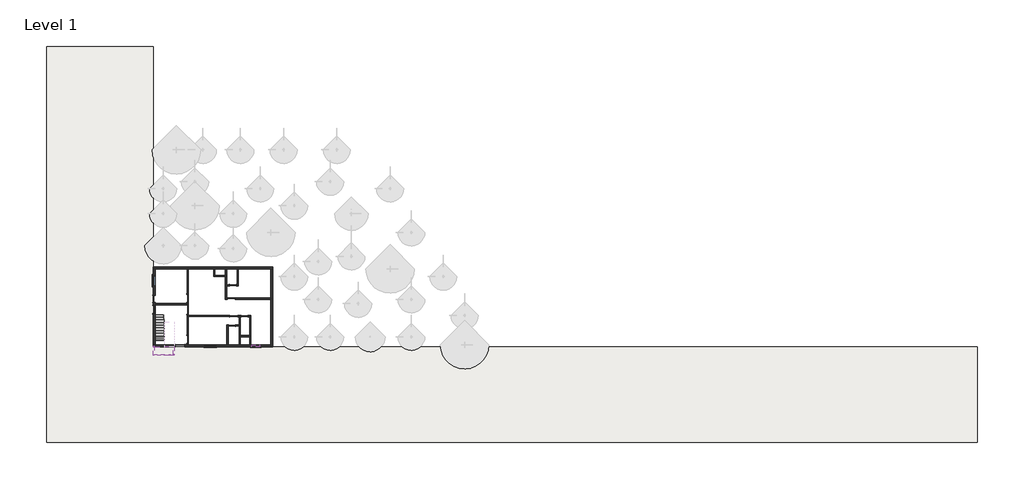
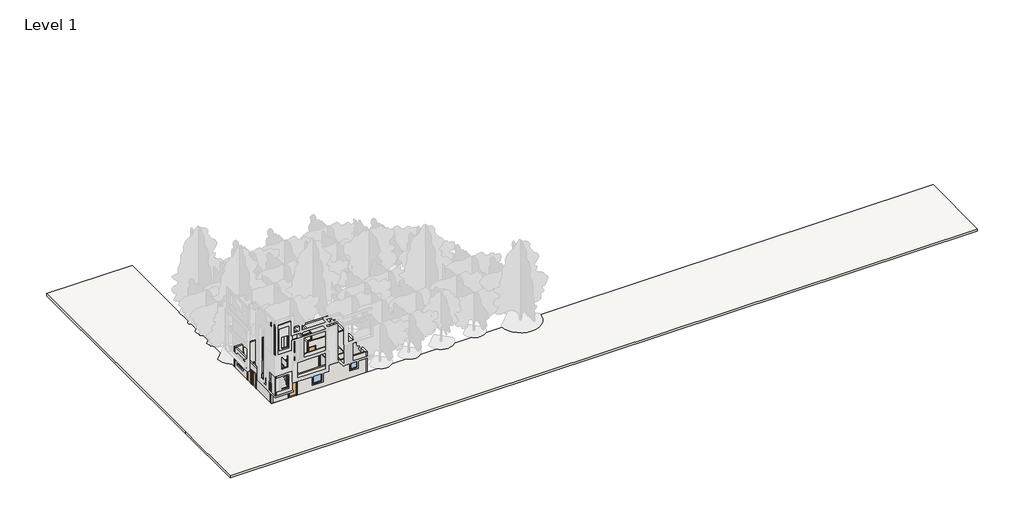
# One storey, part 1 of 2: 24 walls, 11 doors, 4 windows, 2 slabs, 1 stair flight.
"""IFC4 building model written with IfcOpenShell, lengths in millimetres."""

from ifc_helpers import new_model, si_unit, frame, origin, origin_with_axes, place, context, project, spatial, polyline, outline, extrude, faceted_brep, transform, mapped, element, save
from components import door_1fe7f57d, door_85036156, door_a3eb833a, door_a1797ceb, door_a90ba1ad, door_4f94b823, door_0848dd25, window_6c5853a0, window_f887c457, window_76f305d9

model = new_model("IFC4")

# Units and contexts
model_context = context("Model", 3, world=origin())
ifc_project = project(units=[si_unit("LENGTHUNIT", "METRE", prefix="MILLI")], contexts=[model_context])

# Site, building, storey
site = spatial("IfcSite", under=ifc_project)
building = spatial("IfcBuilding", under=site)
storey = spatial("IfcBuildingStorey", under=building, Name="Level 1", Elevation=0.0)

# Doors
placement = place(None, origin())
door_shape = door_1fe7f57d(model_context)
element("IfcDoor", 1, ObjectType="Single-Flush : 30\" x 80\"", at=placement, inside=storey, context=model_context, shape_type="MappedRepresentation", body=[
    mapped(door_shape, transform((-1197.7394758, 10653.5495492, 0.0), x_axis=(1.0, 0.0, 0.0), y_axis=(0.0, 1.0, 0.0), z_axis=(0.0, 0.0, 1.0))),
])
element("IfcDoor", 2, ObjectType="Single-Flush : 30\" x 80\"", at=placement, inside=storey, context=model_context, shape_type="MappedRepresentation", body=[
    mapped(door_shape, transform((135.7605242, 7148.3495492, 0.0), x_axis=(-1.0, 0.0, 0.0), y_axis=(0.0, -1.0, 0.0), z_axis=(0.0, 0.0, 1.0))),
])
element("IfcDoor", 3, ObjectType="Single-Flush : 30\" x 80\"", at=placement, inside=storey, context=model_context, shape_type="MappedRepresentation", body=[
    mapped(door_shape, transform((-1324.7394758, 6056.1495492, 0.0), x_axis=(-1.0, 0.0, 0.0), y_axis=(0.0, -1.0, 0.0), z_axis=(0.0, 0.0, 1.0))),
])
door_2_shape = door_85036156(model_context)
element("IfcDoor", 4, ObjectType="Single-Flush : 30\" x 80\"", at=placement, inside=storey, context=model_context, shape_type="MappedRepresentation", body=[
    mapped(door_2_shape, transform((-10227.4394758, 9091.4495492, 0.0), x_axis=(0.0, -1.0, 0.0), y_axis=(1.0, 0.0, 0.0), z_axis=(0.0, 0.0, 1.0))),
])
door_3_shape = door_a3eb833a(model_context)
element("IfcDoor", 5, ObjectType="Single-Flush : 36\" x 84\"", at=placement, inside=storey, context=model_context, shape_type="MappedRepresentation", body=[
    mapped(door_3_shape, transform((-6392.0394758, 9167.6495492, 0.0), x_axis=(0.0, 1.0, 0.0), y_axis=(-1.0, 0.0, 0.0), z_axis=(0.0, 0.0, 1.0))),
])
element("IfcDoor", 6, ObjectType="Single-Flush : 36\" x 84\"", at=placement, inside=storey, context=model_context, shape_type="MappedRepresentation", body=[
    mapped(door_3_shape, transform((-1400.9394758, 9129.5495492, 0.0), x_axis=(-1.0, 0.0, 0.0), y_axis=(0.0, -1.0, 0.0), z_axis=(0.0, 0.0, 1.0))),
])
element("IfcDoor", 7, ObjectType="Single-Flush : 36\" x 84\"", at=placement, inside=storey, context=model_context, shape_type="MappedRepresentation", body=[
    mapped(door_3_shape, transform((-1083.4394758, 7148.3495492, 0.0), x_axis=(1.0, 0.0, 0.0), y_axis=(0.0, 1.0, 0.0), z_axis=(0.0, 0.0, 1.0))),
])
door_4_shape = door_a1797ceb(model_context)
element("IfcDoor", 8, ObjectType="Single-Flush : 36\" x 84\"", at=placement, inside=storey, context=model_context, shape_type="MappedRepresentation", body=[
    mapped(door_4_shape, transform((-6392.0394758, 4468.6495492, 0.0), x_axis=(0.0, -1.0, 0.0), y_axis=(1.0, 0.0, 0.0), z_axis=(0.0, 0.0, 1.0))),
])
door_5_shape = door_a90ba1ad(model_context)
element("IfcDoor", 9, ObjectType="Single-Flush : 36\" x 84\"", at=placement, inside=storey, context=model_context, shape_type="MappedRepresentation", body=[
    mapped(door_5_shape, transform((-10227.4394758, 7872.2495492, 0.0), x_axis=(0.0, 1.0, 0.0), y_axis=(-1.0, 0.0, 0.0), z_axis=(0.0, 0.0, 1.0))),
])
door_6_shape = door_4f94b823(model_context)
element("IfcDoor", 10, ObjectType="Single-Flush : 42\" x 84\" 3,6\"", at=placement, inside=storey, context=model_context, shape_type="MappedRepresentation", body=[
    mapped(door_6_shape, transform((-6392.0394758, 7872.2495492, 0.0), x_axis=(0.0, -1.0, 0.0), y_axis=(1.0, 0.0, 0.0), z_axis=(0.0, 0.0, 1.0))),
])
door_7_shape = door_0848dd25(model_context)
element("IfcDoor", 11, ObjectType="Single-Flush : 42\" x 84\" 3,6\"", at=placement, inside=storey, context=model_context, shape_type="MappedRepresentation", body=[
    mapped(door_7_shape, transform((-7268.3394758, 3744.7495492, 0.0), x_axis=(-1.0, 0.0, 0.0), y_axis=(0.0, -1.0, 0.0), z_axis=(0.0, 0.0, 1.0))),
])

# Slabs
element("IfcSlab", 12, ObjectType="8\" Thickness", at=placement, inside=storey, context=model_context, shape_type="Brep", body=[
    faceted_brep([(-10341.7394758, 3630.4495492, 1741.7142857), (-10341.7394758, 2639.8495492, 1741.7142857), (-7928.7394758, 2639.8495492, 1741.7142857), (-7928.7394758, 3630.4495492, 1741.7142857), (-7928.7394758, 3649.4995492, 1741.7142857), (-8995.5394758, 3649.4995492, 1741.7142857), (-8995.5394758, 3630.4495492, 1741.7142857), (-9044.7519758, 3630.4495492, 1741.7142857), (-9044.7519758, 3519.3245492, 1741.7142857), (-10114.7269758, 3519.3245492, 1741.7142857), (-10114.7269758, 3630.4495492, 1741.7142857), (-10341.7394758, 3630.4495492, 1538.5142857), (-10341.7394758, 2639.8495492, 1538.5142857), (-7928.7394758, 2639.8495492, 1538.5142857), (-10114.7269758, 3630.4495492, 1538.5142857), (-10114.7269758, 3620.9245492, 1538.5142857), (-9044.7519758, 3620.9245492, 1538.5142857), (-9044.7519758, 3630.4495492, 1538.5142857), (-8995.5394758, 3630.4495492, 1538.5142857), (-8995.5394758, 3649.4995492, 1538.5142857), (-7928.7394758, 3649.4995492, 1538.5142857), (-7928.7394758, 3630.4495492, 1538.5142857), (-10114.7269758, 3519.3245492, 1630.5892857), (-9044.7519758, 3519.3245492, 1630.5892857), (-9044.7519758, 3620.9245492, 1630.5892857), (-10114.7269758, 3620.9245492, 1630.5892857)], [[[0, 1, 2, 3, 4, 5, 6, 7, 8, 9, 10]], [[1, 0, 11, 12]], [[2, 1, 12, 13]], [[12, 11, 14, 15, 16, 17, 18, 19, 20, 21, 13]], [[3, 2, 13, 21]], [[5, 4, 20, 19]], [[6, 18, 17, 7]], [[22, 23, 24, 25]], [[9, 22, 25, 15, 14, 10]], [[23, 22, 9, 8]], [[23, 8, 7, 17, 16, 24]], [[25, 24, 16, 15]], [[11, 0, 10, 14]], [[4, 3, 21, 20]], [[6, 5, 19, 18]]]),
])
element("IfcSlab", 13, ObjectType="Generic - 12\"", at=placement, inside=storey, context=model_context, shape_type="SweptSolid", body=[
    extrude(outline(polyline([(-10341.7394758, 3630.4495492), (84024.3724501, 3630.4495492), (84024.3724501, -7342.3504508), (-22533.7394758, -7342.3504508), (-22533.7394758, 3630.4495492), (-22533.7394758, 38026.55562), (-10341.7394758, 38026.55562), (-10341.7394758, 3630.4495492)])), frame((0.0, 0.0, -311.15), z_axis=(0.0, 0.0, 1.0), x_axis=(1.0, 0.0, 0.0)), (0.0, 0.0, 1.0), 304.8),
])

# Stair flight
element("IfcStairFlight", 14, ObjectType="3/4\" Nosing 6 1/2\" Depth", at=placement, inside=storey, context=model_context, shape_type="Brep", body=[
    faceted_brep([(-10113.1394758, 7288.0495492, 145.1428571), (-9046.3394758, 7288.0495492, 145.1428571), (-9046.3394758, 7268.9995492, 0.0), (-10113.1394758, 7268.9995492, 0.0), (-10113.1394758, 6964.1995492, 145.1428571), (-9046.3394758, 6964.1995492, 145.1428571), (-9046.3394758, 6964.1995492, 0.0), (-10113.1394758, 6964.1995492, 0.0), (-9046.3394758, 6983.2495492, 290.2857143), (-10113.1394758, 6983.2495492, 290.2857143), (-10113.1394758, 6659.3995492, 290.2857143), (-9046.3394758, 6659.3995492, 290.2857143), (-9046.3394758, 6659.3995492, 107.422474), (-9046.3394758, 6884.9867446, 0.0), (-10113.1394758, 6884.9867446, 0.0), (-10113.1394758, 6659.3995492, 107.422474), (-9046.3394758, 6678.4495492, 435.4285714), (-10113.1394758, 6678.4495492, 435.4285714), (-10113.1394758, 6354.5995492, 435.4285714), (-9046.3394758, 6354.5995492, 435.4285714), (-9046.3394758, 6354.5995492, 252.5653311), (-10113.1394758, 6354.5995492, 252.5653311), (-9046.3394758, 6373.6495492, 580.5714286), (-10113.1394758, 6373.6495492, 580.5714286), (-10113.1394758, 6049.7995492, 580.5714286), (-9046.3394758, 6049.7995492, 580.5714286), (-9046.3394758, 6049.7995492, 397.7081883), (-10113.1394758, 6049.7995492, 397.7081883), (-9046.3394758, 6068.8495492, 725.7142857), (-10113.1394758, 6068.8495492, 725.7142857), (-10113.1394758, 5744.9995492, 725.7142857), (-9046.3394758, 5744.9995492, 725.7142857), (-9046.3394758, 5744.9995492, 542.8510454), (-10113.1394758, 5744.9995492, 542.8510454), (-9046.3394758, 5764.0495492, 870.8571429), (-10113.1394758, 5764.0495492, 870.8571429), (-10113.1394758, 5440.1995492, 870.8571429), (-9046.3394758, 5440.1995492, 870.8571429), (-9046.3394758, 5440.1995492, 687.9939026), (-10113.1394758, 5440.1995492, 687.9939026), (-9046.3394758, 5459.2495492, 1016.0), (-10113.1394758, 5459.2495492, 1016.0), (-10113.1394758, 5135.3995492, 1016.0), (-9046.3394758, 5135.3995492, 1016.0), (-9046.3394758, 5135.3995492, 833.1367597), (-10113.1394758, 5135.3995492, 833.1367597), (-9046.3394758, 5154.4495492, 1161.1428571), (-10113.1394758, 5154.4495492, 1161.1428571), (-10113.1394758, 4830.5995492, 1161.1428571), (-9046.3394758, 4830.5995492, 1161.1428571), (-9046.3394758, 4830.5995492, 978.2796169), (-10113.1394758, 4830.5995492, 978.2796169), (-9046.3394758, 4849.6495492, 1306.2857143), (-10113.1394758, 4849.6495492, 1306.2857143), (-10113.1394758, 4525.7995492, 1306.2857143), (-9046.3394758, 4525.7995492, 1306.2857143), (-9046.3394758, 4525.7995492, 1123.422474), (-10113.1394758, 4525.7995492, 1123.422474), (-9046.3394758, 4544.8495492, 1451.4285714), (-10113.1394758, 4544.8495492, 1451.4285714), (-10113.1394758, 4220.9995492, 1451.4285714), (-9046.3394758, 4220.9995492, 1451.4285714), (-9046.3394758, 4220.9995492, 1268.5653311), (-10113.1394758, 4220.9995492, 1268.5653311), (-9046.3394758, 4240.0495492, 1596.5714286), (-10113.1394758, 4240.0495492, 1596.5714286), (-10113.1394758, 3916.1995492, 1596.5714286), (-9046.3394758, 3916.1995492, 1596.5714286), (-9046.3394758, 3916.1995492, 1413.7081883), (-10113.1394758, 3916.1995492, 1413.7081883), (-9046.3394758, 3935.2495492, 1741.7142857), (-10113.1394758, 3935.2495492, 1741.7142857), (-10113.1394758, 3528.8495492, 1741.7142857), (-9046.3394758, 3528.8495492, 1741.7142857), (-9046.3394758, 3528.8495492, 1640.1142857), (-9046.3394758, 3630.4495492, 1640.1142857), (-9046.3394758, 3630.4495492, 1538.5142857), (-9046.3394758, 3654.1067446, 1538.5142857), (-10113.1394758, 3654.1067446, 1538.5142857), (-10113.1394758, 3630.4495492, 1538.5142857), (-10113.1394758, 3630.4495492, 1640.1142857), (-10113.1394758, 3528.8495492, 1640.1142857)], [[[0, 1, 2, 3]], [[1, 0, 4, 5]], [[1, 5, 6, 2]], [[4, 0, 3, 7]], [[8, 9, 10, 11]], [[6, 5, 8, 11, 12, 13]], [[4, 7, 14, 15, 10, 9]], [[5, 4, 9, 8]], [[16, 17, 18, 19]], [[16, 19, 20, 12, 11]], [[18, 17, 10, 15, 21]], [[11, 10, 17, 16]], [[22, 23, 24, 25]], [[22, 25, 26, 20, 19]], [[24, 23, 18, 21, 27]], [[19, 18, 23, 22]], [[28, 29, 30, 31]], [[28, 31, 32, 26, 25]], [[30, 29, 24, 27, 33]], [[25, 24, 29, 28]], [[34, 35, 36, 37]], [[34, 37, 38, 32, 31]], [[36, 35, 30, 33, 39]], [[31, 30, 35, 34]], [[40, 41, 42, 43]], [[40, 43, 44, 38, 37]], [[42, 41, 36, 39, 45]], [[37, 36, 41, 40]], [[46, 47, 48, 49]], [[46, 49, 50, 44, 43]], [[48, 47, 42, 45, 51]], [[43, 42, 47, 46]], [[52, 53, 54, 55]], [[52, 55, 56, 50, 49]], [[54, 53, 48, 51, 57]], [[49, 48, 53, 52]], [[58, 59, 60, 61]], [[58, 61, 62, 56, 55]], [[60, 59, 54, 57, 63]], [[55, 54, 59, 58]], [[64, 65, 66, 67]], [[64, 67, 68, 62, 61]], [[66, 65, 60, 63, 69]], [[61, 60, 65, 64]], [[70, 71, 72, 73]], [[67, 70, 73, 74, 75, 76, 77, 68]], [[72, 71, 66, 69, 78, 79, 80, 81]], [[79, 76, 75, 80]], [[67, 66, 71, 70]], [[2, 6, 13, 14, 7, 3]], [[77, 78, 69, 63, 57, 51, 45, 39, 33, 27, 21, 15, 14, 13, 12, 20, 26, 32, 38, 44, 50, 56, 62, 68]], [[81, 80, 75, 74]], [[81, 74, 73, 72]], [[78, 77, 76, 79]]]),
])

# Walls
element("IfcWall", 15, ObjectType="Generic - 5\"", at=placement, inside=storey, context=model_context, shape_type="Brep", body=[
    faceted_brep([(-6328.5394758, 4925.8495492, 0.0), (-6328.5394758, 7084.8495492, 0.0), (-6328.5394758, 7211.8495492, 0.0), (-6328.5394758, 7338.8495492, 0.0), (-6328.5394758, 7338.8495492, 2133.6), (-6328.5394758, 8405.6495492, 2133.6), (-6328.5394758, 8405.6495492, 0.0), (-6328.5394758, 8710.4495492, 0.0), (-6328.5394758, 8710.4495492, 2133.6), (-6328.5394758, 9624.8495492, 2133.6), (-6328.5394758, 9624.8495492, 0.0), (-6328.5394758, 12545.8495492, 0.0), (-6328.5394758, 12545.8495492, 3048.0), (-6328.5394758, 7211.8495492, 3048.0), (-6328.5394758, 7084.8495492, 3048.0), (-6328.5394758, 3859.0495492, 3048.0), (-6328.5394758, 3859.0495492, 0.0), (-6328.5394758, 4011.4495492, 0.0), (-6328.5394758, 4011.4495492, 2133.6), (-6328.5394758, 4925.8495492, 2133.6), (-6455.5394758, 7338.8495492, 2133.6), (-6455.5394758, 7338.8495492, 0.0), (-6455.5394758, 4925.8495492, 0.0), (-6455.5394758, 4925.8495492, 2133.6), (-6455.5394758, 4011.4495492, 2133.6), (-6455.5394758, 4011.4495492, 0.0), (-6455.5394758, 3859.0495492, 0.0), (-6455.5394758, 3859.0495492, 3048.0), (-6455.5394758, 8431.0495492, 3048.0), (-6455.5394758, 8558.0495492, 3048.0), (-6455.5394758, 12545.8495492, 3048.0), (-6455.5394758, 12545.8495492, 0.0), (-6455.5394758, 9624.8495492, 0.0), (-6455.5394758, 9624.8495492, 2133.6), (-6455.5394758, 8710.4495492, 2133.6), (-6455.5394758, 8710.4495492, 0.0), (-6455.5394758, 8558.0495492, 0.0), (-6455.5394758, 8431.0495492, 0.0), (-6455.5394758, 8405.6495492, 0.0), (-6455.5394758, 8405.6495492, 2133.6)], [[[0, 1, 2, 3, 4, 5, 6, 7, 8, 9, 10, 11, 12, 13, 14, 15, 16, 17, 18, 19]], [[20, 21, 22, 23, 24, 25, 26, 27, 28, 29, 30, 31, 32, 33, 34, 35, 36, 37, 38, 39]], [[11, 10, 32, 31]], [[26, 25, 17, 16]], [[22, 21, 3, 2, 1, 0]], [[38, 37, 36, 35, 7, 6]], [[15, 14, 13, 12, 30, 29, 28, 27]], [[16, 15, 27, 26]], [[12, 11, 31, 30]], [[33, 32, 10, 9]], [[34, 33, 9, 8]], [[35, 34, 8, 7]], [[18, 17, 25, 24]], [[19, 18, 24, 23]], [[0, 19, 23, 22]], [[4, 3, 21, 20]], [[5, 4, 20, 39]], [[6, 5, 39, 38]]]),
])
element("IfcWall", 16, ObjectType="Generic - 5\"", at=placement, inside=storey, context=model_context, shape_type="SweptSolid", body=[
    extrude(outline(polyline([(-10113.1394758, 8558.0495492), (-6455.5394758, 8558.0495492), (-6455.5394758, 8431.0495492), (-10113.1394758, 8431.0495492), (-10113.1394758, 8558.0495492)])), origin_with_axes(), (0.0, 0.0, 1.0), 3048.0),
])
element("IfcWall", 17, ObjectType="Generic - 5\"", at=placement, inside=storey, context=model_context, shape_type="Brep", body=[
    faceted_brep([(-245.2394758, 7211.8495492, 2032.0), (-245.2394758, 7211.8495492, 0.0), (-626.2394758, 7211.8495492, 0.0), (-626.2394758, 7211.8495492, 2133.6), (-1540.6394758, 7211.8495492, 2133.6), (-1540.6394758, 7211.8495492, 0.0), (-6328.5394758, 7211.8495492, 0.0), (-6328.5394758, 7211.8495492, 3048.0), (719.9605242, 7211.8495492, 3048.0), (719.9605242, 7211.8495492, 0.0), (516.7605242, 7211.8495492, 0.0), (516.7605242, 7211.8495492, 2032.0), (-626.2394758, 7084.8495492, 0.0), (-473.8394758, 7084.8495492, 0.0), (-346.8394758, 7084.8495492, 0.0), (-245.2394758, 7084.8495492, 0.0), (-245.2394758, 7084.8495492, 2032.0), (516.7605242, 7084.8495492, 2032.0), (516.7605242, 7084.8495492, 0.0), (719.9605242, 7084.8495492, 0.0), (719.9605242, 7084.8495492, 3048.0), (-346.8394758, 7084.8495492, 3048.0), (-473.8394758, 7084.8495492, 3048.0), (-6328.5394758, 7084.8495492, 3048.0), (-6328.5394758, 7084.8495492, 0.0), (-1540.6394758, 7084.8495492, 0.0), (-1540.6394758, 7084.8495492, 2133.6), (-626.2394758, 7084.8495492, 2133.6)], [[[0, 1, 2, 3, 4, 5, 6, 7, 8, 9, 10, 11]], [[12, 13, 14, 15, 16, 17, 18, 19, 20, 21, 22, 23, 24, 25, 26, 27]], [[25, 24, 6, 5]], [[10, 9, 19, 18]], [[2, 1, 15, 14, 13, 12]], [[8, 7, 23, 22, 21, 20]], [[7, 6, 24, 23]], [[9, 8, 20, 19]], [[3, 2, 12, 27]], [[4, 3, 27, 26]], [[5, 4, 26, 25]], [[16, 15, 1, 0]], [[17, 16, 0, 11]], [[18, 17, 11, 10]]]),
])
element("IfcWall", 18, ObjectType="Generic - 5\"", at=placement, inside=storey, context=model_context, shape_type="Brep", body=[
    faceted_brep([(-2061.3394758, 11656.8495492, 0.0), (-2061.3394758, 9066.0495492, 0.0), (-2061.3394758, 9066.0495492, 3048.0), (-2061.3394758, 11656.8495492, 3048.0), (-1934.3394758, 11656.8495492, 0.0), (-1934.3394758, 11656.8495492, 3048.0), (-1934.3394758, 10717.0495492, 3048.0), (-1934.3394758, 10590.0495492, 3048.0), (-1934.3394758, 9193.0495492, 3048.0), (-1934.3394758, 9066.0495492, 3048.0), (-1934.3394758, 9066.0495492, 0.0), (-1934.3394758, 9193.0495492, 0.0), (-1934.3394758, 10590.0495492, 0.0), (-1934.3394758, 10717.0495492, 0.0)], [[[0, 1, 2, 3]], [[4, 5, 6, 7, 8, 9, 10, 11, 12, 13]], [[1, 0, 4, 13, 12, 11, 10]], [[2, 1, 10, 9]], [[3, 2, 9, 8, 7, 6, 5]], [[0, 3, 5, 4]]]),
])
element("IfcWall", 19, ObjectType="Generic - 5\"", at=placement, inside=storey, context=model_context, shape_type="SweptSolid", body=[
    extrude(outline(polyline([(0.0, -1934.3394758), (0.0, -1858.1394758), (2133.6, -1858.1394758), (2133.6, -943.7394758), (0.0, -943.7394758), (0.0, 3145.6605242), (3048.0, 3145.6605242), (3048.0, -1934.3394758), (0.0, -1934.3394758)])), frame((0.0, 9066.0495492, 0.0), z_axis=(0.0, 1.0, 0.0), x_axis=(0.0, 0.0, 1.0)), (0.0, 0.0, 1.0), 127.0),
])
element("IfcWall", 20, ObjectType="Generic - 5\"", at=placement, inside=storey, context=model_context, shape_type="Brep", body=[
    faceted_brep([(-346.8394758, 3859.0495492, 0.0), (-346.8394758, 4773.4495492, 0.0), (-346.8394758, 4900.4495492, 0.0), (-346.8394758, 7084.8495492, 0.0), (-346.8394758, 7084.8495492, 3048.0), (-346.8394758, 4900.4495492, 3048.0), (-346.8394758, 4773.4495492, 3048.0), (-346.8394758, 3859.0495492, 3048.0), (-473.8394758, 3859.0495492, 0.0), (-473.8394758, 3859.0495492, 3048.0), (-473.8394758, 5992.6495492, 3048.0), (-473.8394758, 6119.6495492, 3048.0), (-473.8394758, 7084.8495492, 3048.0), (-473.8394758, 7084.8495492, 0.0), (-473.8394758, 6119.6495492, 0.0), (-473.8394758, 5992.6495492, 0.0)], [[[0, 1, 2, 3, 4, 5, 6, 7]], [[8, 9, 10, 11, 12, 13, 14, 15]], [[3, 2, 1, 0, 8, 15, 14, 13]], [[7, 6, 5, 4, 12, 11, 10, 9]], [[4, 3, 13, 12]], [[0, 7, 9, 8]]]),
])
element("IfcWall", 21, ObjectType="Generic - 5\"", at=placement, inside=storey, context=model_context, shape_type="Brep", body=[
    faceted_brep([(846.9605242, 3859.0495492, 0.0), (846.9605242, 7211.8495492, 0.0), (846.9605242, 7211.8495492, 3048.0), (846.9605242, 3859.0495492, 3048.0), (719.9605242, 3859.0495492, 0.0), (719.9605242, 3859.0495492, 3048.0), (719.9605242, 4773.4495492, 3048.0), (719.9605242, 4900.4495492, 3048.0), (719.9605242, 7084.8495492, 3048.0), (719.9605242, 7211.8495492, 3048.0), (719.9605242, 7211.8495492, 0.0), (719.9605242, 7084.8495492, 0.0), (719.9605242, 4900.4495492, 0.0), (719.9605242, 4773.4495492, 0.0)], [[[0, 1, 2, 3]], [[4, 5, 6, 7, 8, 9, 10, 11, 12, 13]], [[1, 0, 4, 13, 12, 11, 10]], [[3, 2, 9, 8, 7, 6, 5]], [[0, 3, 5, 4]], [[2, 1, 10, 9]]]),
])
element("IfcWall", 22, ObjectType="Generic - 5\"", at=placement, inside=storey, context=model_context, shape_type="Brep", body=[
    faceted_brep([(-1756.5394758, 3859.0495492, 0.0), (-1756.5394758, 5992.6495492, 0.0), (-1756.5394758, 6119.6495492, 0.0), (-1756.5394758, 6119.6495492, 3048.0), (-1756.5394758, 5992.6495492, 3048.0), (-1756.5394758, 3859.0495492, 3048.0), (-1883.5394758, 3859.0495492, 0.0), (-1883.5394758, 3859.0495492, 3048.0), (-1883.5394758, 6119.6495492, 3048.0), (-1883.5394758, 6119.6495492, 0.0)], [[[0, 1, 2, 3, 4, 5]], [[6, 7, 8, 9]], [[2, 1, 0, 6, 9]], [[5, 4, 3, 8, 7]], [[0, 5, 7, 6]], [[3, 2, 9, 8]]]),
])
element("IfcWall", 23, ObjectType="Generic - 5\"", at=placement, inside=storey, context=model_context, shape_type="SweptSolid", body=[
    extrude(outline(polyline([(0.0, -1756.5394758), (0.0, -1705.7394758), (2032.0, -1705.7394758), (2032.0, -943.7394758), (0.0, -943.7394758), (0.0, -473.8394758), (3048.0, -473.8394758), (3048.0, -1756.5394758), (0.0, -1756.5394758)])), frame((0.0, 5992.6495492, 0.0), z_axis=(0.0, 1.0, 0.0), x_axis=(0.0, 0.0, 1.0)), (0.0, 0.0, 1.0), 127.0),
])
element("IfcWall", 24, ObjectType="Generic - 5\"", at=placement, inside=storey, context=model_context, shape_type="SweptSolid", body=[
    extrude(outline(polyline([(719.9605242, 4773.4495492), (-346.8394758, 4773.4495492), (-346.8394758, 4900.4495492), (719.9605242, 4900.4495492), (719.9605242, 4773.4495492)])), origin_with_axes(), (0.0, 0.0, 1.0), 3048.0),
])
element("IfcWall", 25, ObjectType="Generic - 5\"", at=placement, inside=storey, context=model_context, shape_type="Brep", body=[
    faceted_brep([(-715.1394758, 12545.8495492, 0.0), (-715.1394758, 10717.0495492, 0.0), (-715.1394758, 10590.0495492, 0.0), (-715.1394758, 10590.0495492, 3048.0), (-715.1394758, 10717.0495492, 3048.0), (-715.1394758, 12545.8495492, 3048.0), (-588.1394758, 12545.8495492, 0.0), (-588.1394758, 12545.8495492, 3048.0), (-588.1394758, 10590.0495492, 3048.0), (-588.1394758, 10590.0495492, 0.0)], [[[0, 1, 2, 3, 4, 5]], [[6, 7, 8, 9]], [[2, 1, 0, 6, 9]], [[5, 4, 3, 8, 7]], [[0, 5, 7, 6]], [[3, 2, 9, 8]]]),
])
element("IfcWall", 26, ObjectType="Generic - 5\"", at=placement, inside=storey, context=model_context, shape_type="SweptSolid", body=[
    extrude(outline(polyline([(2032.0, -816.7394758), (0.0, -816.7394758), (0.0, -715.1394758), (3048.0, -715.1394758), (3048.0, -1934.3394758), (0.0, -1934.3394758), (0.0, -1578.7394758), (2032.0, -1578.7394758), (2032.0, -816.7394758)])), frame((0.0, 10590.0495492, 0.0), z_axis=(0.0, 1.0, 0.0), x_axis=(0.0, 0.0, 1.0)), (0.0, 0.0, 1.0), 127.0),
])
element("IfcWall", 27, ObjectType="Generic - 5\"", at=placement, inside=storey, context=model_context, shape_type="Brep", body=[
    faceted_brep([(-3407.5394758, 12545.8495492, 0.0), (-3407.5394758, 11656.8495492, 0.0), (-3407.5394758, 11656.8495492, 3048.0), (-3407.5394758, 12545.8495492, 3048.0), (-3280.5394758, 12545.8495492, 0.0), (-3280.5394758, 12545.8495492, 3048.0), (-3280.5394758, 11783.8495492, 3048.0), (-3280.5394758, 11656.8495492, 3048.0), (-3280.5394758, 11656.8495492, 0.0), (-3280.5394758, 11783.8495492, 0.0)], [[[0, 1, 2, 3]], [[4, 5, 6, 7, 8, 9]], [[1, 0, 4, 9, 8]], [[3, 2, 7, 6, 5]], [[0, 3, 5, 4]], [[2, 1, 8, 7]]]),
])
element("IfcWall", 28, ObjectType="Generic - 5\"", at=placement, inside=storey, context=model_context, shape_type="Brep", body=[
    faceted_brep([(-2061.3394758, 11656.8495492, 914.4), (-3280.5394758, 11656.8495492, 914.4), (-3280.5394758, 11656.8495492, 0.0), (-2061.3394758, 11656.8495492, 0.0), (-1934.3394758, 11656.8495492, 0.0), (-1934.3394758, 11656.8495492, 3048.0), (-2061.3394758, 11656.8495492, 3048.0), (-3280.5394758, 11656.8495492, 3048.0), (-3280.5394758, 11656.8495492, 2133.6), (-2061.3394758, 11656.8495492, 2133.6), (-3280.5394758, 11783.8495492, 0.0), (-3280.5394758, 11783.8495492, 914.4), (-2061.3394758, 11783.8495492, 914.4), (-2061.3394758, 11783.8495492, 2133.6), (-3280.5394758, 11783.8495492, 2133.6), (-3280.5394758, 11783.8495492, 3048.0), (-2061.3394758, 11783.8495492, 3048.0), (-1934.3394758, 11783.8495492, 3048.0), (-1934.3394758, 11783.8495492, 0.0), (-2061.3394758, 11783.8495492, 0.0)], [[[0, 1, 2, 3, 4, 5, 6, 7, 8, 9]], [[10, 11, 12, 13, 14, 15, 16, 17, 18, 19]], [[4, 3, 2, 10, 19, 18]], [[7, 6, 5, 17, 16, 15]], [[8, 7, 15, 14]], [[2, 1, 11, 10]], [[5, 4, 18, 17]], [[12, 11, 1, 0]], [[13, 12, 0, 9]], [[14, 13, 9, 8]]]),
])
element("IfcWall", 29, ObjectType="Generic - 5\"", at=placement, inside=storey, context=model_context, shape_type="SweptSolid", body=[
    extrude(outline(polyline([(-1934.3394758, 12545.8495492), (-1934.3394758, 11783.8495492), (-2061.3394758, 11783.8495492), (-2061.3394758, 12545.8495492), (-1934.3394758, 12545.8495492)])), origin_with_axes(), (0.0, 0.0, 1.0), 3048.0),
])
element("IfcWall", 30, ObjectType="Generic - 5\"", at=placement, inside=storey, context=model_context, shape_type="Brep", body=[
    faceted_brep([(-10341.7394758, 3630.4495492, 9144.0), (-10341.7394758, 3630.4495492, 6096.0), (-10341.7394758, 3630.4495492, 3048.0), (-10341.7394758, 3630.4495492, 1538.5142857), (-10341.7394758, 2639.8495492, 1538.5142857), (-10341.7394758, 2639.8495492, 12192.0), (-10341.7394758, 3744.7495492, 12192.0), (-10341.7394758, 3744.7495492, 9144.0), (-10214.7394758, 3630.4495492, 1538.5142857), (-10214.7394758, 3630.4495492, 9144.0), (-10214.7394758, 3744.7495492, 9144.0), (-10214.7394758, 3744.7495492, 12192.0), (-10214.7394758, 2766.8495492, 12192.0), (-10214.7394758, 2639.8495492, 12192.0), (-10214.7394758, 2639.8495492, 1538.5142857), (-10214.7394758, 2766.8495492, 1538.5142857)], [[[0, 1, 2, 3, 4, 5, 6, 7]], [[8, 9, 10, 11, 12, 13, 14, 15]], [[4, 3, 8, 15, 14]], [[6, 5, 13, 12, 11]], [[5, 4, 14, 13]], [[7, 6, 11, 10]], [[7, 10, 9, 0]], [[0, 9, 8, 3, 2, 1]]]),
])
element("IfcWall", 31, ObjectType="Generic - 5\"", at=placement, inside=storey, context=model_context, shape_type="Brep", body=[
    faceted_brep([(-10214.7394758, 2639.8495492, 1538.5142857), (-7928.7394758, 2639.8495492, 1538.5142857), (-7928.7394758, 2639.8495492, 3048.0), (-7928.7394758, 2639.8495492, 6096.0), (-7928.7394758, 2639.8495492, 9144.0), (-7928.7394758, 2639.8495492, 10363.2), (-7928.7394758, 2639.8495492, 12192.0), (-10214.7394758, 2639.8495492, 12192.0), (-9478.1394758, 2639.8495492, 4267.2), (-8563.7394758, 2639.8495492, 4267.2), (-8563.7394758, 2639.8495492, 2438.4), (-9478.1394758, 2639.8495492, 2438.4), (-9478.1394758, 2639.8495492, 7315.2), (-8563.7394758, 2639.8495492, 7315.2), (-8563.7394758, 2639.8495492, 5486.4), (-9478.1394758, 2639.8495492, 5486.4), (-9478.1394758, 2639.8495492, 10363.2), (-8563.7394758, 2639.8495492, 10363.2), (-8563.7394758, 2639.8495492, 8534.4), (-9478.1394758, 2639.8495492, 8534.4), (-10214.7394758, 2766.8495492, 1538.5142857), (-10214.7394758, 2766.8495492, 12192.0), (-7928.7394758, 2766.8495492, 12192.0), (-7928.7394758, 2766.8495492, 10363.2), (-7928.7394758, 2766.8495492, 9144.0), (-7928.7394758, 2766.8495492, 7634.5142857), (-7928.7394758, 2766.8495492, 3048.0), (-7928.7394758, 2766.8495492, 1538.5142857), (-8055.7394758, 2766.8495492, 1538.5142857), (-9478.1394758, 2766.8495492, 4267.2), (-9478.1394758, 2766.8495492, 2438.4), (-8563.7394758, 2766.8495492, 2438.4), (-8563.7394758, 2766.8495492, 4267.2), (-9478.1394758, 2766.8495492, 7315.2), (-9478.1394758, 2766.8495492, 5486.4), (-8563.7394758, 2766.8495492, 5486.4), (-8563.7394758, 2766.8495492, 7315.2), (-9478.1394758, 2766.8495492, 10363.2), (-9478.1394758, 2766.8495492, 8534.4), (-8563.7394758, 2766.8495492, 8534.4), (-8563.7394758, 2766.8495492, 10363.2)], [[[0, 1, 2, 3, 4, 5, 6, 7], [8, 9, 10, 11], [12, 13, 14, 15], [16, 17, 18, 19]], [[20, 21, 22, 23, 24, 25, 26, 27, 28], [29, 30, 31, 32], [33, 34, 35, 36], [37, 38, 39, 40]], [[1, 0, 20, 28, 27]], [[7, 6, 22, 21]], [[0, 7, 21, 20]], [[1, 27, 26, 25, 24, 23, 22, 6, 5, 4, 3, 2]], [[30, 29, 8, 11]], [[31, 30, 11, 10]], [[32, 31, 10, 9]], [[29, 32, 9, 8]], [[34, 33, 12, 15]], [[35, 34, 15, 14]], [[36, 35, 14, 13]], [[33, 36, 13, 12]], [[38, 37, 16, 19]], [[39, 38, 19, 18]], [[40, 39, 18, 17]], [[37, 40, 17, 16]]]),
])
element("IfcWall", 32, ObjectType="Generic - 5\"", at=placement, inside=storey, context=model_context, shape_type="Brep", body=[
    faceted_brep([(-7928.7394758, 2766.8495492, 1538.5142857), (-7928.7394758, 3630.4495492, 1538.5142857), (-7928.7394758, 3630.4495492, 3048.0), (-7928.7394758, 2766.8495492, 3048.0), (-8055.7394758, 2766.8495492, 1538.5142857), (-8055.7394758, 2766.8495492, 3048.0), (-8055.7394758, 3630.4495492, 3048.0), (-8055.7394758, 3630.4495492, 1538.5142857), (-7992.2394758, 3630.4495492, 1538.5142857)], [[[0, 1, 2, 3]], [[4, 5, 6, 7]], [[1, 0, 4, 7, 8]], [[3, 2, 6, 5]], [[2, 1, 8, 7, 6]], [[0, 3, 5, 4]]]),
])
element("IfcWall", 33, ObjectType="Generic - 9\"", at=placement, inside=storey, context=model_context, shape_type="Brep", body=[
    faceted_brep([(-10341.7394758, 12545.8495492, 0.0), (-10113.1394758, 12545.8495492, 0.0), (-6455.5394758, 12545.8495492, 0.0), (-6328.5394758, 12545.8495492, 0.0), (-3407.5394758, 12545.8495492, 0.0), (-3280.5394758, 12545.8495492, 0.0), (-2061.3394758, 12545.8495492, 0.0), (-1934.3394758, 12545.8495492, 0.0), (-715.1394758, 12545.8495492, 0.0), (-588.1394758, 12545.8495492, 0.0), (3145.6605242, 12545.8495492, 0.0), (3374.2605242, 12545.8495492, 0.0), (3374.2605242, 12545.8495492, 3048.0), (3145.6605242, 12545.8495492, 3048.0), (-588.1394758, 12545.8495492, 3048.0), (-715.1394758, 12545.8495492, 3048.0), (-1934.3394758, 12545.8495492, 3048.0), (-2061.3394758, 12545.8495492, 3048.0), (-3280.5394758, 12545.8495492, 3048.0), (-3407.5394758, 12545.8495492, 3048.0), (-6328.5394758, 12545.8495492, 3048.0), (-6455.5394758, 12545.8495492, 3048.0), (-10113.1394758, 12545.8495492, 3048.0), (-10341.7394758, 12545.8495492, 3048.0), (-10341.7394758, 12774.4495492, 0.0), (-10341.7394758, 12774.4495492, 3048.0), (3374.2605242, 12774.4495492, 3048.0), (3374.2605242, 12774.4495492, 0.0)], [[[0, 1, 2, 3, 4, 5, 6, 7, 8, 9, 10, 11, 12, 13, 14, 15, 16, 17, 18, 19, 20, 21, 22, 23]], [[24, 25, 26, 27]], [[11, 10, 9, 8, 7, 6, 5, 4, 3, 2, 1, 0, 24, 27]], [[23, 22, 21, 20, 19, 18, 17, 16, 15, 14, 13, 12, 26, 25]], [[12, 11, 27, 26]], [[0, 23, 25, 24]]]),
])
element("IfcWall", 34, ObjectType="Generic - 9\"", at=placement, inside=storey, context=model_context, shape_type="Brep", body=[
    faceted_brep([(3145.6605242, 12545.8495492, 0.0), (3145.6605242, 9193.0495492, 0.0), (3145.6605242, 9066.0495492, 0.0), (3145.6605242, 3859.0495492, 0.0), (3145.6605242, 3630.4495492, 0.0), (3145.6605242, 3630.4495492, 3048.0), (3145.6605242, 3859.0495492, 3048.0), (3145.6605242, 9066.0495492, 3048.0), (3145.6605242, 9193.0495492, 3048.0), (3145.6605242, 12545.8495492, 3048.0), (3374.2605242, 12545.8495492, 0.0), (3374.2605242, 12545.8495492, 3048.0), (3374.2605242, 3630.4495492, 3048.0), (3374.2605242, 3630.4495492, 0.0)], [[[0, 1, 2, 3, 4, 5, 6, 7, 8, 9]], [[10, 11, 12, 13]], [[4, 3, 2, 1, 0, 10, 13]], [[9, 8, 7, 6, 5, 12, 11]], [[0, 9, 11, 10]], [[5, 4, 13, 12]]]),
])
element("IfcWall", 35, ObjectType="Generic - 9\"", at=placement, inside=storey, context=model_context, shape_type="Brep", body=[
    faceted_brep([(-7801.7394758, 3859.0495492, 2133.6), (-7801.7394758, 3859.0495492, 0.0), (-7992.2394758, 3859.0495492, 0.0), (-7992.2394758, 3859.0495492, 1538.5142857), (-8055.7394758, 3859.0495492, 1538.5142857), (-8055.7394758, 3859.0495492, 3048.0), (-6455.5394758, 3859.0495492, 3048.0), (-6328.5394758, 3859.0495492, 3048.0), (-1883.5394758, 3859.0495492, 3048.0), (-1756.5394758, 3859.0495492, 3048.0), (-473.8394758, 3859.0495492, 3048.0), (-346.8394758, 3859.0495492, 3048.0), (719.9605242, 3859.0495492, 3048.0), (846.9605242, 3859.0495492, 3048.0), (3145.6605242, 3859.0495492, 3048.0), (3145.6605242, 3859.0495492, 0.0), (846.9605242, 3859.0495492, 0.0), (719.9605242, 3859.0495492, 0.0), (-346.8394758, 3859.0495492, 0.0), (-473.8394758, 3859.0495492, 0.0), (-1756.5394758, 3859.0495492, 0.0), (-1883.5394758, 3859.0495492, 0.0), (-6328.5394758, 3859.0495492, 0.0), (-6455.5394758, 3859.0495492, 0.0), (-6734.9394758, 3859.0495492, 0.0), (-6734.9394758, 3859.0495492, 2133.6), (948.5605242, 3859.0495492, 2133.6), (948.5605242, 3859.0495492, 1219.2), (1862.9605242, 3859.0495492, 1219.2), (1862.9605242, 3859.0495492, 2133.6), (-4398.1394758, 3859.0495492, 2133.6), (-4398.1394758, 3859.0495492, 914.4), (-3178.9394758, 3859.0495492, 914.4), (-3178.9394758, 3859.0495492, 2133.6), (-7992.2394758, 3630.4495492, 0.0), (-7801.7394758, 3630.4495492, 0.0), (-7801.7394758, 3630.4495492, 2133.6), (-6734.9394758, 3630.4495492, 2133.6), (-6734.9394758, 3630.4495492, 0.0), (3145.6605242, 3630.4495492, 0.0), (3145.6605242, 3630.4495492, 3048.0), (-7928.7394758, 3630.4495492, 3048.0), (-8055.7394758, 3630.4495492, 3048.0), (-8055.7394758, 3630.4495492, 1538.5142857), (-7992.2394758, 3630.4495492, 1538.5142857), (948.5605242, 3630.4495492, 2133.6), (1862.9605242, 3630.4495492, 2133.6), (1862.9605242, 3630.4495492, 1219.2), (948.5605242, 3630.4495492, 1219.2), (-4398.1394758, 3630.4495492, 2133.6), (-3178.9394758, 3630.4495492, 2133.6), (-3178.9394758, 3630.4495492, 914.4), (-4398.1394758, 3630.4495492, 914.4)], [[[0, 1, 2, 3, 4, 5, 6, 7, 8, 9, 10, 11, 12, 13, 14, 15, 16, 17, 18, 19, 20, 21, 22, 23, 24, 25], [26, 27, 28, 29], [30, 31, 32, 33]], [[34, 35, 36, 37, 38, 39, 40, 41, 42, 43, 44], [45, 46, 47, 48], [49, 50, 51, 52]], [[2, 1, 35, 34]], [[24, 23, 22, 21, 20, 19, 18, 17, 16, 15, 39, 38]], [[14, 13, 12, 11, 10, 9, 8, 7, 6, 5, 42, 41, 40]], [[15, 14, 40, 39]], [[3, 2, 34, 44]], [[43, 4, 3, 44]], [[5, 4, 43, 42]], [[27, 26, 45, 48]], [[28, 27, 48, 47]], [[29, 28, 47, 46]], [[26, 29, 46, 45]], [[31, 30, 49, 52]], [[32, 31, 52, 51]], [[33, 32, 51, 50]], [[30, 33, 50, 49]], [[36, 35, 1, 0]], [[37, 36, 0, 25]], [[38, 37, 25, 24]]]),
])
element("IfcWall", 36, ObjectType="Generic - 9\"", at=placement, inside=storey, context=model_context, shape_type="Brep", body=[
    faceted_brep([(-10113.1394758, 8329.4495492, 2133.6), (-10113.1394758, 8329.4495492, 0.0), (-10113.1394758, 8431.0495492, 0.0), (-10113.1394758, 8558.0495492, 0.0), (-10113.1394758, 8710.4495492, 0.0), (-10113.1394758, 8710.4495492, 2032.0), (-10113.1394758, 9472.4495492, 2032.0), (-10113.1394758, 9472.4495492, 0.0), (-10113.1394758, 12545.8495492, 0.0), (-10113.1394758, 12545.8495492, 3048.0), (-10113.1394758, 9472.4495492, 3048.0), (-10113.1394758, 8710.4495492, 3048.0), (-10113.1394758, 8558.0495492, 3048.0), (-10113.1394758, 8431.0495492, 3048.0), (-10113.1394758, 6030.7495492, 3048.0), (-10113.1394758, 6030.7495492, 2438.4), (-10113.1394758, 5116.3495492, 2438.4), (-10113.1394758, 5116.3495492, 3048.0), (-10113.1394758, 3859.0495492, 3048.0), (-10113.1394758, 3859.0495492, 0.0), (-10113.1394758, 7415.0495492, 0.0), (-10113.1394758, 7415.0495492, 2133.6), (-10113.1394758, 11783.8495492, 2133.6), (-10113.1394758, 11783.8495492, 914.4), (-10113.1394758, 10564.6495492, 914.4), (-10113.1394758, 10564.6495492, 2133.6), (-10341.7394758, 8710.4495492, 0.0), (-10341.7394758, 8329.4495492, 0.0), (-10341.7394758, 8329.4495492, 2133.6), (-10341.7394758, 7415.0495492, 2133.6), (-10341.7394758, 7415.0495492, 0.0), (-10341.7394758, 3859.0495492, 0.0), (-10341.7394758, 3859.0495492, 3048.0), (-10341.7394758, 5116.3495492, 3048.0), (-10341.7394758, 5116.3495492, 2438.4), (-10341.7394758, 6030.7495492, 2438.4), (-10341.7394758, 6030.7495492, 3048.0), (-10341.7394758, 8710.4495492, 3048.0), (-10341.7394758, 9472.4495492, 3048.0), (-10341.7394758, 12545.8495492, 3048.0), (-10341.7394758, 12545.8495492, 0.0), (-10341.7394758, 9472.4495492, 0.0), (-10341.7394758, 9472.4495492, 2032.0), (-10341.7394758, 8710.4495492, 2032.0), (-10341.7394758, 11783.8495492, 2133.6), (-10341.7394758, 10564.6495492, 2133.6), (-10341.7394758, 10564.6495492, 914.4), (-10341.7394758, 11783.8495492, 914.4)], [[[0, 1, 2, 3, 4, 5, 6, 7, 8, 9, 10, 11, 12, 13, 14, 15, 16, 17, 18, 19, 20, 21], [22, 23, 24, 25]], [[26, 27, 28, 29, 30, 31, 32, 33, 34, 35, 36, 37, 38, 39, 40, 41, 42, 43], [44, 45, 46, 47]], [[40, 8, 7, 41]], [[20, 19, 31, 30]], [[4, 3, 2, 1, 27, 26]], [[9, 39, 38, 37, 36, 14, 13, 12, 11, 10]], [[32, 18, 17, 33]], [[9, 8, 40, 39]], [[31, 19, 18, 32]], [[5, 4, 26, 43]], [[6, 5, 43, 42]], [[7, 6, 42, 41]], [[23, 22, 44, 47]], [[24, 23, 47, 46]], [[25, 24, 46, 45]], [[22, 25, 45, 44]], [[35, 15, 14, 36]], [[15, 35, 34, 16]], [[16, 34, 33, 17]], [[28, 27, 1, 0]], [[29, 28, 0, 21]], [[30, 29, 21, 20]]]),
])
element("IfcWall", 37, ObjectType="Generic - 9\"", at=placement, inside=storey, context=model_context, shape_type="Brep", body=[
    faceted_brep([(-10113.1394758, 3859.0495492, 0.0), (-10341.7394758, 3859.0495492, 0.0), (-10341.7394758, 3859.0495492, 3048.0), (-10113.1394758, 3859.0495492, 3048.0), (-10113.1394758, 3859.0495492, 1538.5142857), (-10113.1394758, 3630.4495492, 0.0), (-10113.1394758, 3630.4495492, 1538.5142857), (-10113.1394758, 3630.4495492, 3048.0), (-10341.7394758, 3630.4495492, 3048.0), (-10341.7394758, 3630.4495492, 1538.5142857), (-10341.7394758, 3630.4495492, 0.0)], [[[0, 1, 2, 3, 4]], [[5, 6, 7, 8, 9, 10]], [[1, 0, 5, 10]], [[3, 2, 8, 7]], [[0, 4, 3, 7, 6, 5]], [[1, 10, 9, 8, 2]]]),
])
element("IfcWall", 38, ObjectType="Generic - 9\"", at=placement, inside=storey, context=model_context, shape_type="Brep", body=[
    faceted_brep([(-7992.2394758, 3859.0495492, 0.0), (-10113.1394758, 3859.0495492, 0.0), (-10113.1394758, 3859.0495492, 1538.5142857), (-8055.7394758, 3859.0495492, 1538.5142857), (-7992.2394758, 3859.0495492, 1538.5142857), (-7992.2394758, 3630.4495492, 0.0), (-7992.2394758, 3630.4495492, 1538.5142857), (-8055.7394758, 3630.4495492, 1538.5142857), (-10113.1394758, 3630.4495492, 1538.5142857), (-10113.1394758, 3630.4495492, 0.0)], [[[0, 1, 2, 3, 4]], [[5, 6, 7, 8, 9]], [[1, 0, 5, 9]], [[4, 3, 2, 8, 7, 6]], [[0, 4, 6, 5]], [[2, 1, 9, 8]]]),
])

# Windows
window_shape = window_6c5853a0(model_context)
element("IfcWindow", 39, ObjectType="Fixed : 36\" x 36\"", at=placement, inside=storey, context=model_context, shape_type="MappedRepresentation", body=[
    mapped(window_shape, transform((1367.6605242, 3744.7495492, 304.8), x_axis=(-1.0, 0.0, 0.0), y_axis=(0.0, -1.0, 0.0), z_axis=(0.0, 0.0, 1.0))),
])
window_2_shape = window_f887c457(model_context)
element("IfcWindow", 40, ObjectType="Fixed : 48\" x 48\"", at=placement, inside=storey, context=model_context, shape_type="MappedRepresentation", body=[
    mapped(window_2_shape, transform((-2709.0394758, 11720.3495492, 0.0), x_axis=(-1.0, 0.0, 0.0), y_axis=(0.0, -1.0, 0.0), z_axis=(0.0, 0.0, 1.0))),
])
window_3_shape = window_76f305d9(model_context)
element("IfcWindow", 41, ObjectType="Fixed : 48\" x 48\"", at=placement, inside=storey, context=model_context, shape_type="MappedRepresentation", body=[
    mapped(window_3_shape, transform((-10227.4394758, 11212.3495492, 0.0), x_axis=(0.0, 1.0, 0.0), y_axis=(-1.0, 0.0, 0.0), z_axis=(0.0, 0.0, 1.0))),
])
element("IfcWindow", 42, ObjectType="Fixed : 48\" x 48\"", at=placement, inside=storey, context=model_context, shape_type="MappedRepresentation", body=[
    mapped(window_3_shape, transform((-3826.6394758, 3744.7495492, 0.0), x_axis=(-1.0, 0.0, 0.0), y_axis=(0.0, -1.0, 0.0), z_axis=(0.0, 0.0, 1.0))),
])

save(model, "model.ifc")

# Revit data of these elements
# Type "Single-Flush : 30\" x 80\""
#   Type Mark = "5"
#   Assembly Code = "C1020"
#   Thickness = 0' - 2"
#   Height = 6' - 8"
#   Trim Projection Ext = 0' - 1"
#   Trim Projection Int = 0' - 1"
#   Trim Width = 0' - 3"
#   Width = 2' - 6"
#   Door Material = Door - Panel
#   Frame Material = Door - Frame
#   Function = (empty or 0)
#   Wall Closure = (empty or 0)
# Type "Single-Flush : 36\" x 84\""
#   Type Mark = "1"
#   Assembly Code = "C1020"
#   Thickness = 0' - 2"
#   Height = 7' - 0"
#   Trim Projection Ext = 0' - 1"
#   Trim Projection Int = 0' - 1"
#   Trim Width = 0' - 3"
#   Width = 3' - 0"
#   Door Material = Door - Panel
#   Frame Material = Door - Frame
#   Function = (empty or 0)
#   Wall Closure = (empty or 0)
# Type "Single-Flush : 42\" x 84\" 3,6\""
#   Type Mark = "8"
#   Assembly Code = "C1020"
#   Thickness = 0' - 2"
#   Height = 7' - 0"
#   Trim Projection Ext = 0' - 1"
#   Trim Projection Int = 0' - 1"
#   Trim Width = 0' - 3"
#   Width = 3' - 6"
#   Door Material = Door - Panel
#   Frame Material = Door - Frame
#   Function = (empty or 0)
#   Wall Closure = (empty or 0)
# Type "Generic - 12\""
#   Assembly Code = "B1010"
#   Function = 0
#   Layers, outside or top first: 1' - 0" no material (function 1)
# Type "Generic - 5\""
#   Assembly Code = "B2010"
#   Layers, outside or top first: 0' - 5" no material (function 1)
# Type "Generic - 9\""
#   Assembly Code = "B2010"
#   Layers, outside or top first: 0' - 9" no material (function 1)
# Type "Fixed : 36\" x 36\""
#   Type Mark = "4"
#   Assembly Code = "B2020100"
#   Height = 3' - 0"
#   Default Sill Height = 3' - 0"
#   Width = 3' - 0"
#   Window Inset = 0' - 0 3/4"
#   Glass Pane Material = Glass
#   Sash Material = Sash
#   Wall Closure = (empty or 0)
# Type "Fixed : 48\" x 48\""
#   Type Mark = "2"
#   Assembly Code = "B2020100"
#   Height = 4' - 0"
#   Default Sill Height = 3' - 0"
#   Width = 4' - 0"
#   Window Inset = 0' - 0 3/4"
#   Glass Pane Material = Glass
#   Sash Material = Sash
#   Wall Closure = (empty or 0)
# Elements 1, 2, 3, 4 (IfcDoor, "Single-Flush : 30\" x 80\"")
#   Phase Created = New Construction
#   Materials on its faces: "Door - Frame", "Door - Panel"
# Elements 5, 6, 7, 8, 9 (IfcDoor, "Single-Flush : 36\" x 84\"")
#   Phase Created = New Construction
#   Materials on its faces: "Door - Frame", "Door - Panel"
# Elements 10, 11 (IfcDoor, "Single-Flush : 42\" x 84\" 3,6\"")
#   Phase Created = New Construction
#   Materials on its faces: "Door - Frame", "Door - Panel"
# Element 12 (IfcSlab, "8\" Thickness")
#   Phase Created = New Construction
#   Materials on its faces: "Concrete, Cast-in-Place gray"
# Element 13 (IfcSlab, "Generic - 12\"")
#   built-in parameter 1001955 = 3.14159 (stored number, unit not read)
#   Height Offset From Level = -0' - 0 1/4"
#   Phase Created = New Construction
#   Materials on its faces: "Default Floor", "02 road"
# Element 14 (IfcStairFlight, "3/4\" Nosing 6 1/2\" Depth")
#   Phase Created = New Construction
#   Materials on its faces: "Concrete, Cast-in-Place gray"
# Elements 15, 16, 17, 18, 19, 20, 21, 22, 23, 24, 25, 26, 27, 28, 29 (IfcWall, "Generic - 5\"")
#   Top Offset = 0' - 0"
#   Base Offset = 0' - 0"
#   Unconnected Height = 10' - 0"
#   wall height = 10' - 0"
#   Phase Created = New Construction
#   Base Constraint = Level 1
#   Materials on its faces: "Default Wall"
# Elements 30, 31 (IfcWall, "Generic - 5\"")
#   built-in parameter 1001111 = 5' - 0.57143"
#   Top Offset = 0' - 0"
#   Base Offset = 5' - 0.57143"
#   Unconnected Height = 34' - 11.42857"
#   wall height = 34' - 11.42857"
#   Phase Created = New Construction
#   Base Constraint = Level 1
#   Materials on its faces: "Default Wall", "01 colour 1"
# Element 32 (IfcWall, "Generic - 5\"")
#   built-in parameter 1001111 = 5' - 0.57143"
#   Top Offset = 0' - 0"
#   Base Offset = 5' - 0.57143"
#   Unconnected Height = 4' - 11.42857"
#   wall height = 4' - 11.42857"
#   Phase Created = New Construction
#   Base Constraint = Level 1
#   Materials on its faces: "Default Wall"
# Elements 33, 34 (IfcWall, "Generic - 9\"")
#   Top Offset = 0' - 0"
#   Base Offset = 0' - 0"
#   Unconnected Height = 10' - 0"
#   wall height = 10' - 0"
#   Phase Created = New Construction
#   Base Constraint = Level 1
#   Materials on its faces: "Default Wall", "02 white", "01 colour 1"
# Elements 35, 36, 37 (IfcWall, "Generic - 9\"")
#   Top Offset = 0' - 0"
#   Base Offset = 0' - 0"
#   Unconnected Height = 10' - 0"
#   wall height = 10' - 0"
#   Phase Created = New Construction
#   Base Constraint = Level 1
#   Materials on its faces: "Default Wall", "01 colour 1"
# Element 38 (IfcWall, "Generic - 9\"")
#   Top Offset = 0' - 0"
#   Base Offset = 0' - 0"
#   Unconnected Height = 5' - 0.57143"
#   wall height = 5' - 0.57143"
#   Phase Created = New Construction
#   Base Constraint = Level 1
#   Materials on its faces: "Default Wall", "01 colour 1"
# Element 39 (IfcWindow, "Fixed : 36\" x 36\"")
#   Mark = "22"
#   Phase Created = New Construction
#   Materials on its faces: "Sash", "Glass"
# Element 40 (IfcWindow, "Fixed : 48\" x 48\"")
#   Mark = "1"
#   Phase Created = New Construction
#   Materials on its faces: "Sash", "Glass"
# Element 41 (IfcWindow, "Fixed : 48\" x 48\"")
#   Mark = "17"
#   Phase Created = New Construction
#   Materials on its faces: "Sash", "Glass"
# Element 42 (IfcWindow, "Fixed : 48\" x 48\"")
#   Mark = "21"
#   Phase Created = New Construction
#   Materials on its faces: "Sash", "Glass"
# Materials
#   "Door - Panel": class "Wood", colour RGB 114 82 51, transparency 0
#   "Door - Frame": colour RGB 153 76 43, transparency 0
#   "Glass": class "Glass", colour RGB 218 227 224, transparency 0.85, Description = "Soda Lime Glass", Cost = 0
#   "Sash": class "Wood", colour RGB 136 99 55, transparency 0
#   "Concrete, Cast-in-Place gray": class "Concrete", colour RGB 115 116 108, transparency 0, Description = "Cast-in-place concrete", Cost = 0
#   "Default Floor": colour RGB 80 80 80, transparency 0
#   "02 road": class "Generic", colour RGB 120 120 120, transparency 0, Cost = 0
#   "Default Wall": colour RGB 80 80 80, transparency 0
#   "01 colour 1": class "Generic", colour RGB 120 120 120, transparency 0, Cost = 0
#   "02 white": class "Generic", colour RGB 120 120 120, transparency 0, Cost = 0
